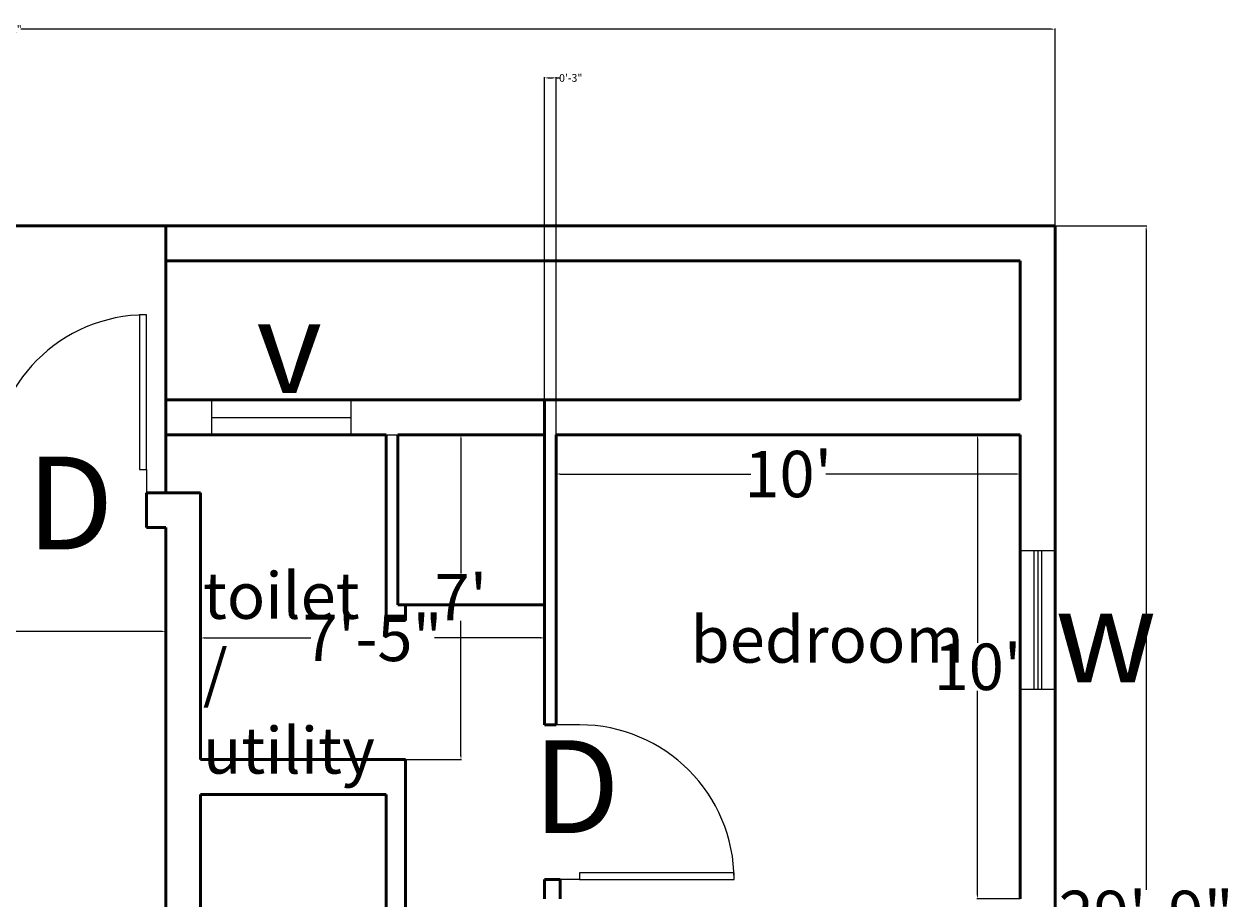
# Model space of a CAD drawing. Units: inches. Extents: x 409 to 7572, y 7 to 725.
# Tile 20 of 38: x 3250 to 3562, y 499 to 725. Entities that reach past the tile are written whole.
import ezdxf

# ---------------------------------------------------------------- set-up
doc = ezdxf.new("R2010")
doc.units = ezdxf.units.IN
doc.header["$MEASUREMENT"] = 0
for name, color, linetype, lineweight in [('A-ANNO-DIMS', 2, 'Continuous', 18), ('A-ANNO-SYMB', 3, 'Continuous', 25), ('A-AREA-IDEN', 7, 'Continuous', 25), ('A-DOOR', 3, 'Continuous', 25), ('A-GLAZ', 4, 'Continuous', 25), ('A-WALL', 7, 'Continuous', 50)]:
    doc.layers.add(name, color=color, linetype=linetype, lineweight=lineweight)
doc.styles.get("Standard").update_dxf_attribs({"font": 'arial.ttf'})
doc.dimstyles.get("Standard").update_dxf_attribs({"dimtxt": 2, "dimasz": 1, "dimexe": 0.18, "dimexo": 0.0625, "dimgap": 0.09, "dimtad": 0, "dimtih": 1, "dimtoh": 1, "dimdec": 0, "dimzin": 0, "dimdsep": 46, "dimlunit": 3, "dimtxsty": 'Standard', "dimcen": 0.09, "dimadec": 0, "dimazin": 0, "dimtfac": 1, "dimtdec": 0, "dimtofl": 0, "dimtmove": 0, "dimatfit": 3, "dimfxl": 1, "dimtolj": 1, "dimtzin": 0, "dimarcsym": 0})

# ---------------------------------------------------------------- blocks, each defined once
blk = doc.blocks.new('*U2')
for p, q in [((0, 0), (0, -6)), ((-40, 0), (-40, -6))]:
    blk.add_line(p, q)
blk.add_lwpolyline([(0, 0), (0, 40), (-1.75, 40), (-1.75, 0)], close=True)
blk.add_arc((0, 0), 40, 90, 180)
blk = doc.blocks.new('*U6')
for p, q in [((0, 0), (0, -6)), ((-40, 0), (-40, -6))]:
    blk.add_line(p, q)
blk.add_lwpolyline([(0, 0), (0, 40), (-1.75, 40), (-1.75, 0)], close=True)
blk.add_arc((0, 0), 40, 90, 180)
blk = doc.blocks.new('*D73')
at = {"layer": 'A-ANNO-DIMS', "color": 0, "lineweight": -2, "transparency": 16777216}
for p, q in [((3388.1, 618.47), (3388.1, 608.19)), ((3508.1, 618.47), (3508.1, 608.19)), ((3389.1, 608.37), (3438.39, 608.37)), ((3507.1, 608.37), (3457.81, 608.37))]:
    blk.add_line(p, q, dxfattribs=at)
at = {"layer": 'A-ANNO-DIMS', "color": 0, "transparency": 16777216}
for points in [[(3389.1, 608.54), (3389.1, 608.2), (3388.1, 608.37)], [(3507.1, 608.54), (3507.1, 608.2), (3508.1, 608.37)]]:
    blk.add_solid(points, dxfattribs=at)
at = {"layer": 'DEFPOINTS', "color": 0, "transparency": 16777216}
for p in [(3388.1, 618.53), (3508.1, 618.53), (3388.1, 608.37)]:
    blk.add_point(p, dxfattribs=at)
at = {"layer": 'A-ANNO-DIMS', "color": 0, "transparency": 16777216, "insert": (3448.1, 608.37), "char_height": 2, "attachment_point": 5}
blk.add_mtext("\\A1;{\\H6x;10'}", dxfattribs=at)
blk = doc.blocks.new('*D74')
at = {"layer": 'A-ANNO-DIMS', "color": 0, "lineweight": -2, "transparency": 16777216}
for p, q in [((3508.04, 618.53), (3496.87, 618.53)), ((3497.05, 617.53), (3497.05, 564.75)), ((3497.05, 499.53), (3497.05, 552.31)), ((3508.04, 498.53), (3496.87, 498.53))]:
    blk.add_line(p, q, dxfattribs=at)
at = {"layer": 'A-ANNO-DIMS', "color": 0, "transparency": 16777216}
for points in [[(3496.88, 617.53), (3497.21, 617.53), (3497.05, 618.53)], [(3496.88, 499.53), (3497.21, 499.53), (3497.05, 498.53)]]:
    blk.add_solid(points, dxfattribs=at)
at = {"layer": 'DEFPOINTS', "color": 0, "transparency": 16777216}
for p in [(3497.05, 618.53), (3508.1, 618.53), (3508.1, 498.53)]:
    blk.add_point(p, dxfattribs=at)
at = {"layer": 'A-ANNO-DIMS', "color": 0, "transparency": 16777216, "insert": (3497.05, 558.53), "char_height": 2, "attachment_point": 5}
blk.add_mtext("\\A1;{\\H6x;10'}", dxfattribs=at)
blk = doc.blocks.new('*D79')
at = {"layer": 'A-ANNO-DIMS', "color": 0, "lineweight": -2, "transparency": 16777216}
for p, q in [((3152.1, 563.4), (3152.1, 567.87)), ((3153.1, 567.69), (3199.46, 567.69)), ((3286.1, 567.69), (3239.73, 567.69)), ((3287.1, 563.4), (3287.1, 567.87))]:
    blk.add_line(p, q, dxfattribs=at)
at = {"layer": 'A-ANNO-DIMS', "color": 0, "transparency": 16777216}
for points in [[(3153.1, 567.86), (3153.1, 567.52), (3152.1, 567.69)], [(3286.1, 567.86), (3286.1, 567.52), (3287.1, 567.69)]]:
    blk.add_solid(points, dxfattribs=at)
at = {"layer": 'DEFPOINTS', "color": 0, "transparency": 16777216}
for p in [(3287.1, 567.69), (3152.1, 563.33), (3287.1, 563.33)]:
    blk.add_point(p, dxfattribs=at)
at = {"layer": 'A-ANNO-DIMS', "color": 0, "transparency": 16777216, "insert": (3219.6, 567.69), "char_height": 2, "attachment_point": 5}
blk.add_mtext('\\A1;{\\H6x;11\'-3"}', dxfattribs=at)
blk = doc.blocks.new('*D85')
at = {"layer": 'A-ANNO-DIMS', "color": 0, "lineweight": -2, "transparency": 16777216}
for p, q in [((3296.1, 568.97), (3296.1, 565.83)), ((3385.1, 568.97), (3385.1, 565.83)), ((3297.1, 566.01), (3324.61, 566.01)), ((3384.1, 566.01), (3356.59, 566.01))]:
    blk.add_line(p, q, dxfattribs=at)
at = {"layer": 'A-ANNO-DIMS', "color": 0, "transparency": 16777216}
for points in [[(3297.1, 566.17), (3297.1, 565.84), (3296.1, 566.01)], [(3384.1, 566.17), (3384.1, 565.84), (3385.1, 566.01)]]:
    blk.add_solid(points, dxfattribs=at)
at = {"layer": 'DEFPOINTS', "color": 0, "transparency": 16777216}
for p in [(3296.1, 569.03), (3385.1, 569.03), (3385.1, 566.01)]:
    blk.add_point(p, dxfattribs=at)
at = {"layer": 'A-ANNO-DIMS', "color": 0, "transparency": 16777216, "insert": (3340.6, 566.01), "char_height": 2, "attachment_point": 5}
blk.add_mtext('\\A1;{\\H6x;7\'-5"}', dxfattribs=at)
blk = doc.blocks.new('*D86')
at = {"layer": 'A-ANNO-DIMS', "color": 0, "lineweight": -2, "transparency": 16777216}
for p, q in [((3315.66, 618.53), (3363.64, 618.53)), ((3363.46, 617.53), (3363.46, 582.62)), ((3363.46, 535.53), (3363.46, 570.44)), ((3315.66, 534.53), (3363.64, 534.53))]:
    blk.add_line(p, q, dxfattribs=at)
at = {"layer": 'A-ANNO-DIMS', "color": 0, "transparency": 16777216}
for points in [[(3363.29, 617.53), (3363.62, 617.53), (3363.46, 618.53)], [(3363.29, 535.53), (3363.62, 535.53), (3363.46, 534.53)]]:
    blk.add_solid(points, dxfattribs=at)
at = {"layer": 'DEFPOINTS', "color": 0, "transparency": 16777216}
for p in [(3315.6, 618.53), (3315.6, 534.53), (3363.46, 534.53)]:
    blk.add_point(p, dxfattribs=at)
at = {"layer": 'A-ANNO-DIMS', "color": 0, "transparency": 16777216, "insert": (3363.46, 576.53), "char_height": 2, "attachment_point": 5}
blk.add_mtext("\\A1;{\\H6x;7'}", dxfattribs=at)
blk = doc.blocks.new('*D90')
at = {"layer": 'A-ANNO-DIMS', "color": 0, "lineweight": -2, "transparency": 16777216}
for p, q in [((2975.1, 672.59), (2975.1, 723.56)), ((2976.1, 723.38), (3242.53, 723.38)), ((3516.1, 723.38), (3249.66, 723.38)), ((3517.1, 672.59), (3517.1, 723.56))]:
    blk.add_line(p, q, dxfattribs=at)
at = {"layer": 'A-ANNO-DIMS', "color": 0, "transparency": 16777216}
for points in [[(2976.1, 723.55), (2976.1, 723.22), (2975.1, 723.38)], [(3516.1, 723.55), (3516.1, 723.22), (3517.1, 723.38)]]:
    blk.add_solid(points, dxfattribs=at)
at = {"layer": 'DEFPOINTS', "color": 0, "transparency": 16777216}
for p in [(2975.1, 723.38), (2975.1, 672.53), (3517.1, 672.53)]:
    blk.add_point(p, dxfattribs=at)
at = {"layer": 'A-ANNO-DIMS', "color": 0, "transparency": 16777216, "insert": (3246.1, 723.38), "char_height": 2, "attachment_point": 5}
blk.add_mtext('\\A1;45\'-2"', dxfattribs=at)
blk = doc.blocks.new('*D92')
at = {"layer": 'A-ANNO-DIMS', "color": 0, "lineweight": -2, "transparency": 16777216}
for p, q in [((3517.16, 672.53), (3540.84, 672.53)), ((3540.66, 671.53), (3540.66, 500.86)), ((3540.66, 316.53), (3540.66, 488.43)), ((3517.16, 315.53), (3540.84, 315.53))]:
    blk.add_line(p, q, dxfattribs=at)
at = {"layer": 'A-ANNO-DIMS', "color": 0, "transparency": 16777216}
for points in [[(3540.5, 671.53), (3540.83, 671.53), (3540.66, 672.53)], [(3540.5, 316.53), (3540.83, 316.53), (3540.66, 315.53)]]:
    blk.add_solid(points, dxfattribs=at)
at = {"layer": 'DEFPOINTS', "color": 0, "transparency": 16777216}
for p in [(3517.1, 672.53), (3540.66, 672.53), (3517.1, 315.53)]:
    blk.add_point(p, dxfattribs=at)
at = {"layer": 'A-ANNO-DIMS', "color": 0, "transparency": 16777216, "insert": (3540.66, 494.65), "char_height": 2, "attachment_point": 5}
blk.add_mtext('\\A1;{\\H6x;29\'-9"}', dxfattribs=at)
blk = doc.blocks.new('WIN-36')
for p, q in [((1699.82, 514.65), (1699.82, 478.65)), ((1700.82, 514.65), (1700.82, 478.65)), ((1701.82, 514.65), (1701.82, 478.65))]:
    blk.add_line(p, q)
blk.add_lwpolyline([(1705.32, 514.65), (1705.32, 478.65), (1696.32, 478.65), (1696.32, 514.65)], close=True)
blk = doc.blocks.new('VENT-36')
blk.add_line((5633.28, 355.73), (5633.28, 391.73))
blk.add_lwpolyline([(5628.78, 355.73), (5628.78, 391.73), (5637.78, 391.73), (5637.78, 355.73)], close=True)
blk = doc.blocks.new('*D185')
at = {"layer": 'A-ANNO-DIMS', "color": 0, "lineweight": -2, "transparency": 16777216}
for p, q in [((3385.1, 627.59), (3385.1, 710.96)), ((3386.1, 710.78), (3387.1, 710.78)), ((3388.1, 618.59), (3388.1, 710.96)), ((3388.1, 710.78), (3389.1, 710.78))]:
    blk.add_line(p, q, dxfattribs=at)
at = {"layer": 'A-ANNO-DIMS', "color": 0, "transparency": 16777216}
for points in [[(3386.1, 710.95), (3386.1, 710.61), (3385.1, 710.78)], [(3387.1, 710.95), (3387.1, 710.61), (3388.1, 710.78)]]:
    blk.add_solid(points, dxfattribs=at)
at = {"layer": 'DEFPOINTS', "color": 0, "transparency": 16777216}
for p in [(3388.1, 710.78), (3385.1, 627.53), (3388.1, 618.53)]:
    blk.add_point(p, dxfattribs=at)
at = {"layer": 'A-ANNO-DIMS', "color": 0, "transparency": 16777216, "insert": (3391.85, 710.78), "char_height": 2, "attachment_point": 5}
blk.add_mtext('\\A1;0\'-3"', dxfattribs=at)

msp = doc.modelspace()

# ---------------------------------------------------------------- linework, layer by layer
at = {"layer": 'A-WALL'}
for p, q in [((3517.1, 672.53), (2975.1, 672.53)), ((3287.1, 672.53), (3287.1, 603.53)), ((3517.1, 315.53), (3517.1, 672.53)), ((3508.1, 663.53), (3287.1, 663.53)), ((3508.1, 627.53), (3508.1, 663.53)), ((3508.1, 627.53), (3287.1, 627.53)), ((3385.1, 627.53), (3385.1, 543.53)), ((3344.1, 618.53), (3287.1, 618.53)), ((3344.1, 618.53), (3344.1, 570.53)), ((3385.1, 618.53), (3347.1, 618.53)), ((3347.1, 618.53), (3347.1, 574.53)), ((3508.1, 618.53), (3388.1, 618.53)), ((3388.1, 618.53), (3388.1, 543.53)), ((3508.1, 498.53), (3508.1, 618.53)), ((3282.1, 603.53), (3296.1, 603.53)), ((3282.1, 603.53), (3282.1, 594.53)), ((3296.1, 603.53), (3296.1, 534.53)), ((3282.1, 594.53), (3287.1, 594.53)), ((3385.1, 574.53), (3347.1, 574.53)), ((3349.1, 574.53), (3349.1, 570.53)), ((3349.1, 570.53), (3344.1, 570.53)), ((3388.1, 543.53), (3385.1, 543.53)), ((3349.1, 534.53), (3296.1, 534.53)), ((3349.1, 534.53), (3349.1, 453.53)), ((3344.1, 525.53), (3296.1, 525.53)), ((3296.1, 525.53), (3296.1, 469.53)), ((3344.1, 525.53), (3344.1, 337.53)), ((3385.1, 498.53), (3385.1, 503.53)), ((3385.1, 503.53), (3389.1, 503.53)), ((3389.1, 503.53), (3389.1, 498.53))]:
    msp.add_line(p, q, dxfattribs=at)
msp.add_lwpolyline([(3287.1, 594.53), (3287.1, 525.53), (3287.1, 469.53)], dxfattribs=at)

# ---------------------------------------------------------------- block references
at = {"layer": 'A-DOOR'}
msp.add_blockref('*U2', (3282.1, 609.53), dxfattribs=at)
at = {"layer": 'A-DOOR', "rotation": 270}
msp.add_blockref('*U6', (3394.1, 503.53), dxfattribs=at)
at = {"layer": 'A-GLAZ', "rotation": 269.9999999999993}
msp.add_blockref('VENT-36', (2943.29, 6256.31), dxfattribs=at)
at = {"layer": 'A-GLAZ'}
msp.add_blockref('WIN-36', (1811.78, 73.99), dxfattribs=at)

# ---------------------------------------------------------------- texts
at = {"layer": 'A-ANNO-SYMB', "char_height": 24, "attachment_point": 1}
for s, width, insert in [('v', 18.2582, (3310.51, 653.33)), ('D', 19.1972, (3251.12, 612.87)), ('w', 18.2582, (3517.1, 578.5)), ('D', 19.1972, (3382.02, 539.54))]:
    msp.add_mtext_dynamic_manual_height_columns(s, width=width, gutter_width=1, heights=[0], dxfattribs=dict(at, insert=insert))
at = {"layer": 'A-AREA-IDEN', "char_height": 12, "attachment_point": 1}
for s, width, insert in [('toilet / utility', 49.2946, (3296.75, 582.94)), ('bedroom', 40.9017, (3422.85, 571.6))]:
    msp.add_mtext_dynamic_manual_height_columns(s, width=width, gutter_width=1, heights=[0], dxfattribs=dict(at, insert=insert))

# ---------------------------------------------------------------- dimensions: what is measured, and where the dimension line sits
at = {"layer": 'A-ANNO-DIMS'}
for base, p1, p2, override, picture, middle in [((2975.1, 723.38), (3517.1, 672.53), (2975.1, 672.53), {"dimclrd": 0, "dimclre": 0, "dimclrt": 0}, '*D90', (3246.1, 723.38)), ((3388.1, 710.78), (3385.1, 627.53), (3388.1, 618.53), {"dimdec": 1, "dimlfac": 1, "dimrnd": 0, "dimzin": 1, "dimdsep": 46, "dimlunit": 4, "dimfrac": 2}, '*D185', (3391.85, 710.78))]:
    dim = msp.add_linear_dim(base=base, p1=p1, p2=p2, dimstyle='Standard', override=override, dxfattribs=at)
    dim.commit()
    dim.dimension.update_dxf_attribs({"geometry": picture, "text_midpoint": middle})
dim = msp.add_linear_dim(base=(3540.66, 672.53), p1=(3517.1, 315.53), p2=(3517.1, 672.53), angle=90, text='{\\H6x;<>}', dimstyle='Standard', override={"dimclrd": 0, "dimclre": 0, "dimclrt": 0}, dxfattribs=at)
dim.commit()
dim.dimension.update_dxf_attribs({"geometry": '*D92', "text_midpoint": (3540.66, 494.65), "dimtype": 160})
for base, p1, p2, picture, middle in [((3363.46, 534.53), (3315.6, 618.53), (3315.6, 534.53), '*D86', (3363.46, 576.53)), ((3497.05, 618.53), (3508.1, 498.53), (3508.1, 618.53), '*D74', (3497.05, 558.53))]:
    dim = msp.add_linear_dim(base=base, p1=p1, p2=p2, angle=90, text='{\\H6x;<>}', dimstyle='Standard', override={"dimclrd": 0, "dimclre": 0, "dimclrt": 0}, dxfattribs=at)
    dim.commit()
    dim.dimension.update_dxf_attribs({"geometry": picture, "text_midpoint": middle})
for base, p1, p2, picture, middle in [((3388.1, 608.37), (3508.1, 618.53), (3388.1, 618.53), '*D73', (3448.1, 608.37)), ((3287.1, 567.69), (3152.1, 563.33), (3287.1, 563.33), '*D79', (3219.6, 567.69)), ((3385.1, 566.01), (3296.1, 569.03), (3385.1, 569.03), '*D85', (3340.6, 566.01))]:
    dim = msp.add_linear_dim(base=base, p1=p1, p2=p2, text='{\\H6x;<>}', dimstyle='Standard', override={"dimclrd": 0, "dimclre": 0, "dimclrt": 0}, dxfattribs=at)
    dim.commit()
    dim.dimension.update_dxf_attribs({"geometry": picture, "text_midpoint": middle})

doc.saveas('drawing.dxf')
